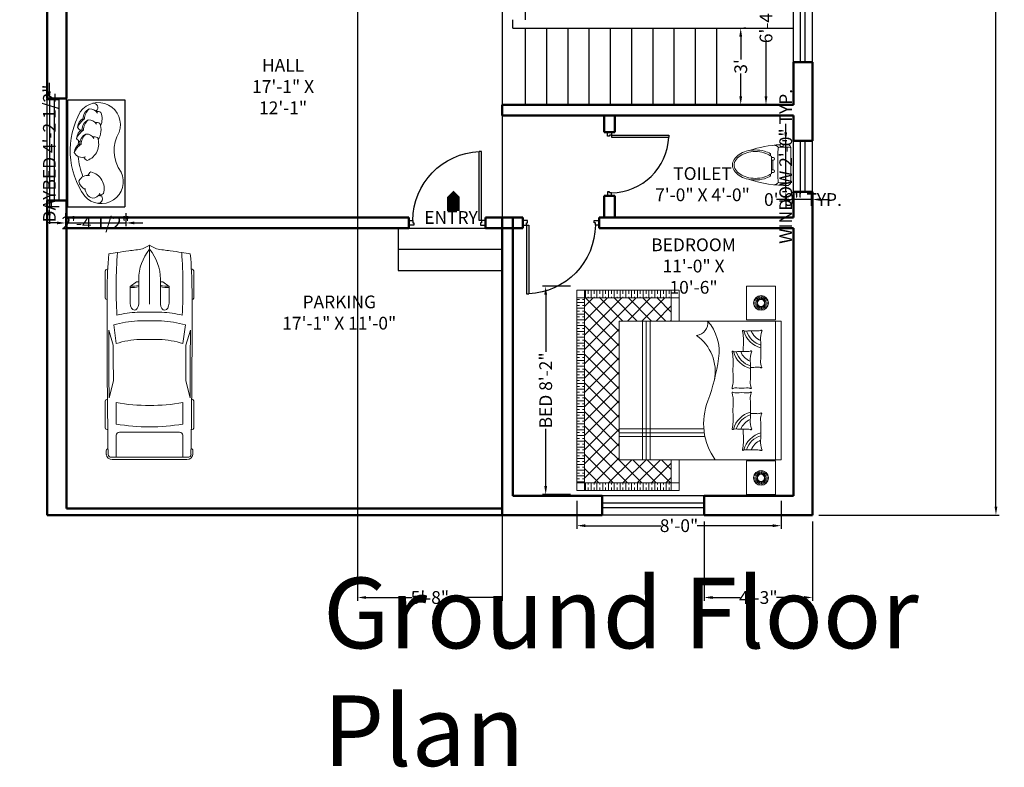
# Model space of a CAD drawing. Units: inches. Extents: x 234 to 707, y 260 to 1025.
# Tile 1 of 3: x 244 to 707, y 260 to 612. Entities that reach past the tile are written whole.
import ezdxf

# ---------------------------------------------------------------- set-up
doc = ezdxf.new("R2010")
doc.units = ezdxf.units.IN
doc.header["$MEASUREMENT"] = 0
for name, color, linetype, lineweight in [('A-ANNO-DIMS', 3, 'Continuous', 18), ('A-ANNO-SYMB', 3, 'Continuous', 18), ('A-ANNO-TEXT', 7, 'Continuous', 35), ('A-AREA-IDEN', 7, 'Continuous', 25), ('A-DOOR', 2, 'Continuous', 25), ('A-FLOR-FIXT', 9, 'Continuous', 18), ('A-FLOR-STRS', 4, 'Continuous', 25), ('A-FURN', 9, 'Continuous', 18), ('A-SITE-VEHI', 8, 'Continuous', 13), ('WALL', 7, 'Continuous', 50), ('WINDOW', 2, 'Continuous', 25)]:
    doc.layers.add(name, color=color, linetype=linetype, lineweight=lineweight)
doc.styles.get("Standard").update_dxf_attribs({"font": 'arial.ttf'})
doc.styles.add('YQ_DIM', font='SUPEROS.SHX', dxfattribs={"width": 0.8, "bigfont": 'HZDX.SHX'})
doc.dimstyles.new('yqi0', dxfattribs={"dimscale": 0, "dimtxt": 6, "dimasz": 4, "dimexe": 1.5, "dimexo": 3, "dimgap": 0.5, "dimtad": 0, "dimdec": 1, "dimdsep": 46, "dimlunit": 4, "dimtxsty": 'Standard', "dimcen": 0, "dimclrd": 256, "dimclre": 256, "dimclrt": 7, "dimadec": 1, "dimazin": 2, "dimtfac": 1, "dimtdec": 1, "dimtix": 1, "dimtmove": 2, "dimatfit": 2, "dimfxl": 1, "dimtolj": 1, "dimtzin": 0, "dimarcsym": 0})

# ---------------------------------------------------------------- blocks, each defined once
blk = doc.blocks.new('*D3')
at = {"layer": 'A-ANNO-DIMS', "color": 0, "lineweight": -2, "transparency": 16777216}
for p, q in [((620.21, 978.74), (705.01, 978.74)), ((703.51, 974.74), (703.51, 684.33)), ((703.51, 382.74), (703.51, 673.15)), ((620.21, 378.74), (705.01, 378.74))]:
    blk.add_line(p, q, dxfattribs=at)
at = {"layer": 'A-ANNO-DIMS', "color": 0, "transparency": 16777216}
for points in [[(702.84, 974.74), (704.17, 974.74), (703.51, 978.74)], [(702.84, 382.74), (704.17, 382.74), (703.51, 378.74)]]:
    blk.add_solid(points, dxfattribs=at)
at = {"layer": 'Defpoints', "color": 0, "transparency": 16777216}
for p in [(617.21, 978.74), (617.21, 378.74), (703.51, 378.74)]:
    blk.add_point(p, dxfattribs=at)
at = {"layer": 'A-ANNO-DIMS', "color": 0, "transparency": 16777216, "insert": (703.51, 678.74), "char_height": 6, "attachment_point": 5, "rotation": 90}
blk.add_mtext("\\A1;50'", dxfattribs=at)
blk = doc.blocks.new('DR_D01')
for p, q in [((-0.45, 0.93), (-0.42, 0.93)), ((-0.45, 0.03), (-0.45, 0.93)), ((-0.42, 0.03), (-0.42, 0.93)), ((-0.5, 0.03), (-0.42, 0.03)), ((-0.5, 0.03), (-0.5, -0.03)), ((-0.45, 0.03), (-0.45, 0)), ((-0.45, 0), (-0.435, 0)), ((-0.435, 0), (-0.435, -0.03)), ((0.435, 0), (0.435, -0.03)), ((0.45, 0), (0.435, 0)), ((0.45, 0.03), (0.45, 0)), ((0.5, 0.03), (0.45, 0.03)), ((0.5, -0.03), (0.5, 0.03)), ((-0.435, -0.03), (-0.5, -0.03)), ((0.435, -0.03), (0.5, -0.03))]:
    blk.add_line(p, q)
blk.add_arc((-0.46, 0.021), 0.91, 0.5915, 87.4664)
blk = doc.blocks.new('WD_WIN4')
for p, q in [((-0.5, 0.5), (0.5, 0.5)), ((-0.5, 0.12), (0.5, 0.12)), ((-0.5, -0.12), (0.5, -0.12)), ((-0.5, -0.5), (0.5, -0.5))]:
    blk.add_line(p, q)
blk = doc.blocks.new('yq_matong_01')
for p, q in [((0, 201), (0, -201)), ((20, 221), (139, 221)), ((252, 138), (252, 114)), ((216, 91), (238, 91)), ((216, 61), (238, 61)), ((223, 61), (223, -61)), ((238, 104), (238, -104)), ((216, -61), (238, -61)), ((216, -91), (238, -91)), ((252, -114), (252, -138)), ((20, -221), (139, -221)), ((97, -221), (97, -226)), ((97, -226), (132, -226)), ((132, -221), (132, -226))]:
    blk.add_line(p, q)
for centre, radius, start, end in [((55, 202), 54.8, 117.322, 181.8992), ((64, -1165), 1417, 71.4068, 91.3856), ((217, 161), 83.2, 95.4963, 139.9324), ((20, 201), 20, 90, 180), ((139, 201), 20, 2.3063, 90), ((-4840, 0), 5003, 357.6937, 2.3063), ((407, -123), 283, 105.2088, 123.2779), ((407, -123), 303, 105.2088, 120.5699), ((439, -242), 427, 74.7912, 105.2088), ((439, -242), 407, 74.7912, 105.2088), ((471, -123), 283, 56.7221, 74.7912), ((471, -123), 303, 56.7221, 74.7912), ((521, -47), 213, 32.2565, 56.7221), ((216, 76), 15, 90, 270), ((357, -47), 193, 123.2779, 128.1384), ((521, -47), 193, 32.2565, 56.7221), ((596, 0), 104, 360, 32.2565), ((596, 0), 124, 360, 32.2565), ((216, -76), 15, 90, 270), ((357, 47), 193, 231.8616, 236.7221), ((407, 123), 283, 236.7221, 254.7912), ((471, 123), 283, 285.2088, 303.2779), ((521, 47), 193, 303.2779, 327.7435), ((521, 47), 213, 303.2779, 327.7435), ((596, 0), 104, 327.7435, 360), ((596, 0), 124, 327.7435, 360), ((51, -204), 51.4, 175.687, 245.0918), ((20, -201), 20, 180, 270), ((157, -247), 63.1, 159.6834, 188.4939), ((72, -247), 63.1, 352.0944, 20.3166), ((64, 1165), 1417, 272.8967, 288.5932), ((139, -201), 20, 270, 357.6937), ((217, -161), 83.2, 220.0676, 264.5037), ((407, 123), 303, 239.4301, 254.7912), ((439, 242), 427, 254.7912, 285.2088), ((439, 242), 407, 254.7912, 285.2088), ((471, 123), 303, 285.2088, 303.2779), ((64, 1165), 1417, 268.6144, 271.2036), ((114, -226), 37, 237.5287, 304.2772)]:
    blk.add_arc(centre, radius, start, end)
blk = doc.blocks.new('20230926_Unit Plans$0$day bed')
blk.add_lwpolyline([(573.063, -307.537, -0.288423), (571.446, -307.621, -0.865931), (571.834, -306.876, 0.308297), (572.6, -306.836, -0.865931)], format="xyb", close=True)
for points in [[(571.715, -307.232, 0.201081), (571.457, -307.227, 0.121523), (571.44, -307.319, -7.115464)], [(571.979, -307.28, 0.24852), (571.668, -307.247, 0.121523), (571.651, -307.338, -7.115464)], [(572.665, -307.475, -0.165541), (572.598, -307.419, -0.425989), (573.013, -307.176, -0.121523), (573.04, -307.265, 7.115464)], [(571.587, -307.568, -0.306663), (571.391, -307.449, -0.30633), (571.474, -307.294, 0.872847)], [(571.798, -307.587, -0.306663), (571.602, -307.468, -0.30633), (571.685, -307.313, 0.872847)], [(572.071, -307.633, -0.306663), (571.875, -307.514, -0.30633), (571.958, -307.359, 0.872847)], [(572.317, -307.553, 0.165541), (572.379, -307.491, 0.425989), (571.941, -307.292, 0.121523), (571.924, -307.384, -7.115464)], [(572.919, -307.529, 0.306663), (573.101, -307.39, 0.30633), (573.003, -307.245, -0.872847)], [(571.743, -307.672, -0.14773), (571.586, -307.542, -0.213343), (571.391, -307.449, -0.178662)], [(571.804, -307.616, -0.116002), (571.743, -307.672, -0.249542), (571.573, -307.568, 9.61688)], [(571.955, -307.691, -0.14773), (571.798, -307.561, -0.213343), (571.602, -307.468, -0.178662)], [(572.019, -307.629, -0.125567), (571.955, -307.691, -0.249542), (571.784, -307.587, 9.61688)], [(572.227, -307.737, -0.14773), (572.07, -307.607, -0.213343), (571.875, -307.514, -0.178662)], [(572.31, -307.523, -0.356772), (572.227, -307.737, -0.249542), (572.057, -307.633, 9.61688)], [(572.669, -307.444, 0.356772), (572.774, -307.648, 0.249542), (572.933, -307.527, -9.61688)]]:
    blk.add_lwpolyline(points, format="xyb")
for centre, radius, start, end in [((573.116, -307.279), 0.084, 357.0539, 145.314), ((572.781, -307.22), 0.275, 348.5451, 359.7611), ((571.366, -307.37), 0.084, 40.6567, 188.9168), ((571.694, -307.277), 0.275, 186.2096, 192.1968), ((572.187, -306.294), 1.371, 274.7225, 291.4116), ((572.187, -306.294), 1.371, 262.2344, 265.3334)]:
    blk.add_arc(centre, radius, start, end)
at = {"layer": 'Defpoints', "ltscale": 0.1, "transparency": 33554687}
for p, q in [((571.219, -306.765), (573.269, -306.765)), ((571.219, -307.865), (571.219, -306.765)), ((573.269, -307.865), (573.269, -306.765)), ((571.219, -307.865), (573.269, -307.865))]:
    blk.add_line(p, q, dxfattribs=at)
blk = doc.blocks.new('*D15')
at = {"layer": 'A-ANNO-DIMS', "color": 0, "lineweight": -2, "transparency": 16777216}
for p, q in [((585.78, 607.74), (584.94, 607.74)), ((583.44, 603.74), (583.44, 593)), ((583.44, 575.74), (583.44, 586.48)), ((585.78, 571.74), (584.94, 571.74))]:
    blk.add_line(p, q, dxfattribs=at)
at = {"layer": 'A-ANNO-DIMS', "color": 0, "transparency": 16777216}
for points in [[(582.77, 603.74), (584.1, 603.74), (583.44, 607.74)], [(582.77, 575.74), (584.1, 575.74), (583.44, 571.74)]]:
    blk.add_solid(points, dxfattribs=at)
at = {"layer": 'Defpoints', "color": 0, "transparency": 16777216}
for p in [(582.78, 607.74), (583.44, 607.74), (582.78, 571.74)]:
    blk.add_point(p, dxfattribs=at)
at = {"layer": 'A-ANNO-DIMS', "color": 0, "transparency": 16777216, "insert": (583.44, 589.74), "char_height": 6, "attachment_point": 5, "rotation": 90}
blk.add_mtext("\\A1;3'", dxfattribs=at)
blk = doc.blocks.new('*D16')
at = {"layer": 'A-ANNO-DIMS', "color": 0, "lineweight": -2, "transparency": 16777216}
for p, q in [((598, 647.74), (596.84, 647.74)), ((595.34, 643.74), (595.34, 618.23)), ((595.34, 575.74), (595.34, 601.25)), ((598, 571.74), (596.84, 571.74))]:
    blk.add_line(p, q, dxfattribs=at)
at = {"layer": 'A-ANNO-DIMS', "color": 0, "transparency": 16777216}
for points in [[(594.67, 643.74), (596, 643.74), (595.34, 647.74)], [(594.67, 575.74), (596, 575.74), (595.34, 571.74)]]:
    blk.add_solid(points, dxfattribs=at)
at = {"layer": 'Defpoints', "color": 0, "transparency": 16777216}
for p in [(595, 647.74), (595.34, 647.74), (595, 571.74)]:
    blk.add_point(p, dxfattribs=at)
at = {"layer": 'A-ANNO-DIMS', "color": 0, "transparency": 16777216, "insert": (595.34, 609.74), "char_height": 6, "attachment_point": 5, "rotation": 90}
blk.add_mtext('\\A1;6\'-4"', dxfattribs=at)
blk = doc.blocks.new('*U19')
for p, q in [((536, 950), (536, 936)), ((1182, 988), (568, 988)), ((1214, 950), (1214, 950)), ((2235, 810), (1899, 912)), ((3412, 904), (3030, 807)), ((3440, 942), (3440, 950)), ((3472, 988), (4087, 988)), ((4119, 950), (4119, 934)), ((1779, 801), (2195, 746)), ((3516, 746), (3994, 746)), ((4179, 670), (4179, -670)), ((4736, 746), (4242, 746)), ((4736, -851), (4736, 851)), ((4785, -832), (4785, 832)), ((756, 241), (1313, 241)), ((816, 241), (816, 283)), ((820, 295), (918, 436)), ((918, 436), (1294, 436)), ((1496, -274), (1496, 274)), ((1690, -267), (1690, 267)), ((4736, -267), (4736, 267)), ((83, 156), (3, 10)), ((2102, 216), (2102, -216)), ((0, 0), (1313, 0)), ((3, -10), (83, -156)), ((756, -241), (1313, -241)), ((816, -241), (816, -283)), ((820, -295), (918, -436)), ((918, -436), (1294, -436)), ((2195, -746), (1779, -801)), ((2235, -810), (1899, -912)), ((3412, -904), (3030, -807)), ((3994, -746), (3516, -746)), ((4242, -746), (4736, -746)), ((536, -950), (536, -936)), ((1182, -988), (568, -988)), ((1214, -950), (1214, -950)), ((3440, -942), (3440, -950)), ((3472, -988), (4087, -988)), ((4119, -950), (4119, -934))]:
    blk.add_line(p, q)
for centre, major_axis, ratio, start_param, end_param in [((6757, -699), (0, 7958), 0.842304, 1.367076, 1.39176), ((1046, -12468), (0, 13417), 0.842304, 0.00281, 0.075598), ((568, 950), (0, -37.6), 0.842304, 3.141593, 4.712389), ((1638, -268113), (0, 269063), 0.842304, -0.013397, 0.002797), ((1182, 950), (0, 37.6), 0.842304, -1.570796, 0), ((1638, -268113), (0, -269025), 0.842304, 3.133765, 3.140441), ((3472, 950), (0, -37.6), 0.842304, 3.141593, 4.712389), ((4087, 950), (0, 37.6), 0.842304, -1.570796, 0), ((4588, 910), (0, 56.4), 0.842304, -0.013017, 1.249894), ((1638, -268131), (0, 269121), 0.842304, -0.013397, -0.013017), ((4673, 851), (0, -75.2), 0.842304, 1.570796, 3.128196), ((4673, 832), (0, -133), 0.842304, 1.570796, 3.128196), ((6583, -699), (0, -7755), 0.842304, 4.528606, 4.561838), ((952, -15087), (0, -15833), 0.842304, 3.096046, 3.200911), ((3414, 137), (0, -2280), 0.842304, 4.449482, 4.652344), ((3436, 137), (0, 2077), 0.842304, 1.245306, 1.50788), ((3800, 71), (0, -2021), 0.842304, 4.372215, 4.640744), ((2433, -93125), (0, -93935), 0.842304, 3.134049, 3.144098), ((434, 0), (0, 3734), 0.842304, 4.511394, 4.913384), ((912, 0), (0, 3734), 0.842304, 4.511394, 4.913384), ((4242, 670), (0, 75.2), 0.842304, 0, 1.570796), ((-5194, 1331), (0, -6374), 0.842304, 1.385369, 1.434372), ((756, -1185), (0, 1427), 0.842304, 0, 0.590319), ((832, 283), (0, 18.8), 0.842304, 0.879714, 1.570796), ((331, 432), (0, 696), 0.842304, 4.435146, 4.718221), ((361, 432), (0, 696), 0.842304, 4.435146, 4.718221), ((1290, 339), (161, -9), 0.603834, -1.395552, 1.581315), ((16, 0), (0, -18.8), 0.842304, 4.131459, 5.293319), ((-5194, -1331), (0, 6374), 0.842304, -1.434372, -1.385369), ((756, 1185), (0, 1427), 0.842304, 2.551274, 3.141593), ((3800, -71), (0, -2021), 0.842304, -1.499151, -1.230623), ((832, -283), (0, -18.8), 0.842304, 4.712389, 5.403472), ((331, -432), (0, -696), 0.842304, 1.564964, 1.848039), ((361, -432), (0, -696), 0.842304, 1.564964, 1.848039), ((3414, -137), (0, -2280), 0.842304, -1.510751, -1.307889), ((3436, -137), (0, -2077), 0.842304, -1.50788, -1.245306), ((6583, 699), (0, 7755), 0.842304, 1.721348, 1.754579), ((6757, 699), (0, 7958), 0.842304, 1.749832, 1.774517), ((952, 15087), (0, -15833), 0.842304, -0.059319, 0.045547), ((2433, 93125), (0, -93935), 0.842304, -0.002505, 0.007544), ((4242, -670), (0, -75.2), 0.842304, 4.712389, 6.283185), ((4673, -851), (0, 75.2), 0.842304, 3.15499, 4.712389), ((4673, -832), (0, -133), 0.842304, 0.013397, 1.570796), ((1046, 12468), (0, -13417), 0.842304, -0.075598, -0.00281), ((568, -950), (0, 37.6), 0.842304, 1.570796, 3.141593), ((1638, 268113), (0, 269063), 0.842304, 3.138796, 3.15499), ((1182, -950), (0, -37.6), 0.842304, 0, 1.570796), ((1638, 268113), (0, -269025), 0.842304, 0.001152, 0.007828), ((3472, -950), (0, -37.6), 0.842304, -1.570796, 0), ((4087, -950), (0, 37.6), 0.842304, 3.141593, 4.712389), ((4588, -910), (0, -56.4), 0.842304, -1.249894, 0.013017), ((1638, 268131), (0, 269121), 0.842304, 3.15461, 3.15499)]:
    blk.add_ellipse(centre, major_axis=major_axis, ratio=ratio, start_param=start_param, end_param=end_param)
at = {"extrusion": (0, 0, -1)}
blk.add_ellipse((1290, -339), major_axis=(161, 9), ratio=0.603834, start_param=-1.395552, end_param=1.581315, dxfattribs=at)
blk = doc.blocks.new('BED')
h = blk.add_hatch()
h.set_pattern_fill('TRANS', color=256, scale=12, style=0)
h.set_pattern_definition([(360, (4433.967, -9715.0492), (1e-15, 3), []), (360, (4433.967, -9713.5492), (1e-15, 3), [1.5, -1.5])])
h.paths.add_polyline_path([(48, -103), (52, -103), (52, -58), (48, -58)])
h.paths.add_polyline_path([(-48, -58), (-52, -58), (-52, -103), (-48, -103)])
h = blk.add_hatch()
h.set_pattern_fill('ANSI37', color=256, scale=42, angle=-90, style=0)
h.set_pattern_definition([(315, (7787.1367, 4477.8466), (3.7123106, 3.7123106), []), (45, (7787.1367, 4477.8466), (-3.7123106, 3.7123106), [])])
h.paths.add_polyline_path([(-36, -85), (-36, -58), (-48, -58), (-48, -103), (48, -103), (48, -58), (36, -58), (36, -85)])
h = blk.add_hatch()
h.set_pattern_fill('TRANS', color=256, scale=12, angle=-90, style=0)
h.set_pattern_definition([(270, (4433.967, -9715.0492), (3, -1e-15), []), (270, (4435.467, -9715.0492), (3, -1e-15), [1.5, -1.5])])
h.paths.add_polyline_path([(48, -107), (48, -103), (-48, -103), (-48, -107)])
for p, q in [((-54, -4), (-54, -19)), ((-36.64, -4), (-54, -4)), ((-36.64, -4), (-36.64, -19)), ((-36, -1), (36, -1)), ((-36, -85), (-36, -1)), ((-36, -4), (36, -4)), ((36, -1), (36, -85)), ((36.64, -4), (36.64, -19)), ((36.64, -4), (54, -4)), ((54, -4), (54, -19)), ((-47.07, -10.7), (-48.9, -9.89)), ((-46.88, -10.37), (-48.5, -9.2)), ((-46.62, -10.08), (-47.96, -8.6)), ((-46.31, -9.86), (-47.31, -8.13)), ((-45.96, -9.7), (-46.58, -7.8)), ((-45.58, -9.62), (-45.8, -7.63)), ((-45.2, -9.62), (-45, -7.63)), ((-44.82, -9.7), (-44.21, -7.79)), ((-44.47, -9.85), (-43.48, -8.12)), ((-44.16, -10.08), (-42.83, -8.59)), ((-43.9, -10.36), (-42.29, -9.18)), ((-43.71, -10.7), (-41.89, -9.88)), ((43.71, -10.7), (41.89, -9.88)), ((43.9, -10.36), (42.29, -9.18)), ((44.16, -10.08), (42.83, -8.59)), ((44.47, -9.85), (43.48, -8.12)), ((44.82, -9.7), (44.21, -7.79)), ((45.2, -9.62), (45, -7.63)), ((45.58, -9.62), (45.8, -7.63)), ((45.96, -9.7), (46.58, -7.8)), ((46.31, -9.86), (47.31, -8.13)), ((46.62, -10.08), (47.96, -8.6)), ((46.88, -10.37), (48.5, -9.2)), ((47.07, -10.7), (48.9, -9.89)), ((-47.23, -11.45), (-49.23, -11.45)), ((-47.19, -11.07), (-49.14, -10.66)), ((-47.19, -11.83), (-49.14, -12.25)), ((-47.07, -12.2), (-48.89, -13.01)), ((-46.87, -12.53), (-48.49, -13.71)), ((-46.62, -12.81), (-47.95, -14.3)), ((-46.3, -13.04), (-47.3, -14.77)), ((-45.95, -13.2), (-46.57, -15.1)), ((-45.58, -13.27), (-45.78, -15.26)), ((-45.19, -13.27), (-44.98, -15.26)), ((-44.82, -13.19), (-44.2, -15.09)), ((-44.47, -13.04), (-43.46, -14.77)), ((-44.16, -12.81), (-42.82, -14.29)), ((-43.9, -12.52), (-42.28, -13.7)), ((-43.71, -12.19), (-41.88, -13)), ((-43.59, -11.06), (-41.64, -10.64)), ((-43.59, -11.83), (-41.63, -12.24)), ((-43.55, -11.44), (-41.55, -11.44)), ((43.55, -11.44), (41.55, -11.44)), ((43.59, -11.83), (41.63, -12.24)), ((43.59, -11.06), (41.64, -10.64)), ((43.71, -12.19), (41.88, -13)), ((43.9, -12.52), (42.28, -13.7)), ((44.16, -12.81), (42.82, -14.29)), ((44.47, -13.04), (43.46, -14.77)), ((44.82, -13.19), (44.2, -15.09)), ((45.19, -13.27), (44.98, -15.26)), ((45.58, -13.27), (45.78, -15.26)), ((45.95, -13.2), (46.57, -15.1)), ((46.3, -13.04), (47.3, -14.77)), ((46.62, -12.81), (47.95, -14.3)), ((46.87, -12.53), (48.49, -13.71)), ((47.07, -12.2), (48.89, -13.01)), ((47.19, -11.07), (49.14, -10.66)), ((47.19, -11.83), (49.14, -12.25)), ((47.23, -11.45), (49.23, -11.45)), ((-36.64, -19), (-54, -19)), ((36.64, -19), (54, -19)), ((24, -85), (24, -40.55)), ((20, -85), (20, -41.14)), ((22, -85), (22, -40.91)), ((-52, -54), (-52, -107)), ((-52, -54), (-36, -54)), ((-48, -54), (-48, -107)), ((36, -54), (52, -54)), ((48, -54), (48, -107)), ((52, -54), (52, -107)), ((-52, -58), (-36, -58)), ((36, -58), (52, -58)), ((36, -69), (-36, -69)), ((36, -71), (-36, -71)), ((36, -73), (-36, -73)), ((36, -85), (-36, -85)), ((-52, -103), (52, -103)), ((-52, -107), (52, -107))]:
    blk.add_line(p, q)
for centre, radius in [((-45.39, -11.45), 3.84), ((-45.39, -11.45), 1.84), ((45.39, -11.45), 3.84), ((45.39, -11.45), 1.84)]:
    blk.add_circle(centre, radius)
for centre, radius, start, end in [((-30.92, -11.24), 0.328, 35.8976, 208.6272), ((-42.38, -17.5), 12.73, 27.1629, 28.6272), ((-44.37, -13.89), 13.5, 357.4804, 9.3956), ((10.15, -16.29), 41.07, 177.4804, 184.5075), ((-33.8, -8.61), 8.46, 289.8695, 338.9843), ((-33.8, -8.61), 12.06, 283.8498, 346.0842), ((-33.8, -8.61), 10.71, 286.0319, 344.1205), ((-26.84, 0.13), 11.82, 251.1782, 273.3982), ((-20.92, -99.64), 88.13, 86.2964, 93.3982), ((-14.79, -4.98), 6.73, 266.2964, 294.303), ((-8.24, -13.16), 3.86, 159.0146, 186.273), ((-36.64, -16.28), 24.71, 358.5721, 6.273), ((-11.92, -11.33), 0.242, 335.7259, 114.303), ((-5.69, -14.14), 6.59, 155.7259, 159.0146), ((11.92, -11.33), 0.242, 65.697, 204.2741), ((5.69, -14.14), 6.59, 20.9854, 24.2741), ((8.24, -13.16), 3.86, 353.727, 20.9854), ((36.64, -16.28), 24.71, 173.727, 181.4279), ((14.79, -4.98), 6.73, 245.697, 273.7036), ((20.92, -99.64), 88.13, 86.6018, 93.7036), ((33.8, -8.61), 12.06, 193.9158, 256.1502), ((33.8, -8.61), 10.71, 195.8795, 253.9681), ((33.8, -8.61), 8.46, 201.0157, 250.1305), ((26.84, 0.13), 11.82, 266.6018, 288.8218), ((30.92, -11.24), 0.328, 331.3728, 144.1024), ((-10.15, -16.29), 41.07, 355.4925, 2.5196), ((44.37, -13.89), 13.5, 170.6044, 182.5196), ((42.38, -17.5), 12.73, 151.3728, 152.8371), ((-32.72, -19.65), 1.93, 327.6219, 339.2246), ((-32.67, -19.67), 1.88, 339.2246, 4.5075), ((-20.16, -16.62), 0.328, 35.8976, 208.6272), ((-31.62, -22.87), 12.73, 27.1629, 28.6272), ((-33.61, -19.26), 13.5, 357.4804, 9.3956), ((-23.04, -13.99), 8.46, 289.8695, 338.9843), ((20.91, -21.66), 41.07, 177.4804, 184.5075), ((-23.04, -13.99), 12.06, 283.8498, 346.0842), ((-23.04, -13.99), 10.71, 286.0319, 344.1205), ((-16.08, -5.24), 11.82, 251.1782, 273.3982), ((-10.15, -105.01), 88.13, 86.2964, 93.3982), ((-4.03, -10.35), 6.73, 266.2964, 294.303), ((2.52, -18.53), 3.86, 159.0146, 186.273), ((-25.88, -21.66), 24.71, 354.3784, 6.273), ((-1.16, -16.7), 0.242, 335.7259, 114.303), ((5.07, -19.51), 6.59, 155.7259, 159.0146), ((1.16, -16.7), 0.242, 65.697, 204.2741), ((-5.07, -19.51), 6.59, 20.9854, 24.2741), ((-2.52, -18.53), 3.86, 353.727, 20.9854), ((25.88, -21.66), 24.71, 173.727, 185.6216), ((4.03, -10.35), 6.73, 245.697, 273.7036), ((10.15, -105.01), 88.13, 86.6018, 93.7036), ((23.04, -13.99), 12.06, 193.9158, 256.1502), ((23.04, -13.99), 10.71, 195.8795, 253.9681), ((23.04, -13.99), 8.46, 201.0157, 250.1305), ((16.08, -5.24), 11.82, 266.6018, 288.8218), ((20.16, -16.62), 0.328, 331.3728, 144.1024), ((-20.91, -21.66), 41.07, 355.4925, 2.5196), ((33.61, -19.26), 13.5, 170.6044, 182.5196), ((31.62, -22.87), 12.73, 151.3728, 152.8371), ((32.67, -19.67), 1.88, 175.4925, 200.7754), ((32.72, -19.65), 1.93, 200.7754, 212.3781), ((-30.88, -20.82), 0.25, 147.6219, 311.9343), ((-25.16, -53.53), 33, 93.5164, 99.6766), ((-25.27, -51.86), 31.33, 86.4836, 93.5164), ((-21.12, 15.68), 36.34, 266.4836, 271.5234), ((-21.91, -25.04), 1.88, 339.2246, 4.5075), ((2.55, -24.46), 3.86, 174.3784, 204.7617), ((-2.55, -24.46), 3.86, 335.2383, 5.6216), ((21.91, -25.04), 1.88, 175.4925, 200.7754), ((21.12, 15.68), 36.34, 268.4766, 273.5164), ((25.27, -51.86), 31.33, 86.4836, 93.5164), ((25.16, -53.53), 33, 80.3234, 86.4836), ((30.88, -20.82), 0.25, 228.0657, 32.3781), ((-20.12, -26.19), 0.25, 147.6219, 311.9343), ((-21.96, -25.02), 1.93, 327.6219, 339.2246), ((-14.4, -58.9), 33, 93.5164, 99.6766), ((-14.51, -57.23), 31.33, 86.4836, 93.5164), ((-10.35, 10.3), 36.34, 266.4836, 275.306), ((-5.78, -38.98), 13.15, 77.9645, 95.306), ((2.5, -0.17), 26.53, 257.9645, 261.9243), ((-1.09, -26.25), 0.228, 231.9005, 52.8902), ((1.09, -26.25), 0.228, 127.1098, 308.0995), ((-2.5, -0.17), 26.53, 278.0757, 282.0355), ((5.78, -38.98), 13.15, 84.694, 102.0355), ((10.35, 10.3), 36.34, 264.694, 273.5164), ((14.51, -57.23), 31.33, 86.4836, 93.5164), ((14.4, -58.9), 33, 80.3234, 86.4836), ((20.12, -26.19), 0.25, 228.0657, 32.3781), ((21.96, -25.02), 1.93, 200.7754, 212.3781), ((-20.27, -56.85), 23.66, 81.0857, 131.6581), ((-9.91, -57.83), 22.61, 78.6456, 145.1521), ((-32.56, -143.87), 111.55, 70.0977, 81.7735), ((17.27, -9.21), 32.05, 248.2778, 305.7663), ((-34.97, -45.63), 6.55, 6.3172, 99.0807)]:
    blk.add_arc(centre, radius, start, end)
blk = doc.blocks.new('*D25')
at = {"layer": 'A-ANNO-DIMS', "lineweight": -2, "transparency": 16777216}
for p, q in [((604.61, 558.74), (604.61, 562.74)), ((605.21, 554.74), (603.11, 554.74)), ((604.61, 530.74), (604.61, 554.74)), ((605.21, 530.74), (603.11, 530.74)), ((604.61, 526.74), (604.61, 522.74))]:
    blk.add_line(p, q, dxfattribs=at)
at = {"layer": 'A-ANNO-DIMS', "transparency": 16777216}
for points in [[(603.95, 558.74), (605.28, 558.74), (604.61, 554.74)], [(603.95, 526.74), (605.28, 526.74), (604.61, 530.74)]]:
    blk.add_solid(points, dxfattribs=at)
at = {"layer": 'Defpoints', "color": 0, "transparency": 16777216}
for p in [(604.61, 554.74), (608.21, 554.74), (608.21, 530.74)]:
    blk.add_point(p, dxfattribs=at)
at = {"layer": 'A-ANNO-DIMS', "color": 7, "transparency": 16777216, "insert": (604.61, 542.74), "char_height": 6, "attachment_point": 5, "rotation": 90}
blk.add_mtext('\\A1;WINDOW 2\'-0" TYP.', dxfattribs=at)
blk = doc.blocks.new('*D26')
at = {"layer": 'A-ANNO-DIMS', "lineweight": -2, "transparency": 16777216}
for p, q in [((604.21, 527.14), (600.21, 527.14)), ((608.21, 527.74), (608.21, 525.64)), ((617.21, 527.14), (608.21, 527.14)), ((617.21, 527.74), (617.21, 525.64)), ((621.21, 527.14), (625.21, 527.14))]:
    blk.add_line(p, q, dxfattribs=at)
at = {"layer": 'A-ANNO-DIMS', "transparency": 16777216}
for points in [[(604.21, 527.81), (604.21, 526.47), (608.21, 527.14)], [(621.21, 527.81), (621.21, 526.47), (617.21, 527.14)]]:
    blk.add_solid(points, dxfattribs=at)
at = {"layer": 'Defpoints', "color": 0, "transparency": 16777216}
for p in [(608.21, 530.74), (617.21, 530.74), (608.21, 527.14)]:
    blk.add_point(p, dxfattribs=at)
at = {"layer": 'A-ANNO-DIMS', "color": 7, "transparency": 16777216, "insert": (612.71, 527.14), "char_height": 6, "attachment_point": 5}
blk.add_mtext('\\A1;0\'-9" TYP.', dxfattribs=at)
blk = doc.blocks.new('*D35')
at = {"layer": 'A-ANNO-DIMS', "lineweight": -2, "transparency": 16777216}
for p, q in [((503.37, 486.32), (490.19, 486.32)), ((491.69, 482.32), (491.69, 455.49)), ((491.69, 392.41), (491.69, 419.24)), ((503.37, 388.41), (490.19, 388.41))]:
    blk.add_line(p, q, dxfattribs=at)
at = {"layer": 'A-ANNO-DIMS', "transparency": 16777216}
for points in [[(491.02, 482.32), (492.35, 482.32), (491.69, 486.32)], [(491.02, 392.41), (492.35, 392.41), (491.69, 388.41)]]:
    blk.add_solid(points, dxfattribs=at)
at = {"layer": 'Defpoints', "color": 0, "transparency": 16777216}
for p in [(506.37, 486.32), (491.69, 388.41), (506.37, 388.41)]:
    blk.add_point(p, dxfattribs=at)
at = {"layer": 'A-ANNO-DIMS', "color": 7, "transparency": 16777216, "insert": (491.69, 437.37), "char_height": 6, "attachment_point": 5, "rotation": 90}
blk.add_mtext('\\A1;BED 8\'-2"', dxfattribs=at)
blk = doc.blocks.new('*D36')
at = {"layer": 'A-ANNO-DIMS', "lineweight": -2, "transparency": 16777216}
for p, q in [((506.37, 385.41), (506.37, 372.23)), ((602.47, 385.41), (602.47, 372.23)), ((510.37, 373.73), (545.94, 373.73)), ((598.47, 373.73), (562.9, 373.73))]:
    blk.add_line(p, q, dxfattribs=at)
at = {"layer": 'A-ANNO-DIMS', "transparency": 16777216}
for points in [[(510.37, 374.39), (510.37, 373.06), (506.37, 373.73)], [(598.47, 374.39), (598.47, 373.06), (602.47, 373.73)]]:
    blk.add_solid(points, dxfattribs=at)
at = {"layer": 'Defpoints', "color": 0, "transparency": 16777216}
for p in [(506.37, 388.41), (602.47, 388.41), (602.47, 373.73)]:
    blk.add_point(p, dxfattribs=at)
at = {"layer": 'A-ANNO-DIMS', "color": 7, "transparency": 16777216, "insert": (554.42, 373.73), "char_height": 6, "attachment_point": 5}
blk.add_mtext('\\A1;8\'-0"', dxfattribs=at)
blk = doc.blocks.new('*D43')
at = {"layer": 'A-ANNO-DIMS', "lineweight": -2, "transparency": 16777216}
for p, q in [((258.2, 577.98), (258.2, 581.98)), ((262.75, 573.98), (256.7, 573.98)), ((258.2, 573.98), (258.2, 523.67)), ((262.75, 523.67), (256.7, 523.67)), ((258.2, 519.67), (258.2, 515.67))]:
    blk.add_line(p, q, dxfattribs=at)
at = {"layer": 'A-ANNO-DIMS', "transparency": 16777216}
for points in [[(257.53, 577.98), (258.86, 577.98), (258.2, 573.98)], [(257.53, 519.67), (258.86, 519.67), (258.2, 523.67)]]:
    blk.add_solid(points, dxfattribs=at)
at = {"layer": 'Defpoints', "color": 0, "transparency": 16777216}
for p in [(265.75, 573.98), (258.2, 523.67), (265.75, 523.67)]:
    blk.add_point(p, dxfattribs=at)
at = {"layer": 'A-ANNO-DIMS', "color": 7, "transparency": 16777216, "insert": (258.2, 548.83), "char_height": 6, "attachment_point": 5, "rotation": 90}
blk.add_mtext('\\A1;DAYBED 4\'-2 1/2"', dxfattribs=at)
blk = doc.blocks.new('*D44')
at = {"layer": 'A-ANNO-DIMS', "lineweight": -2, "transparency": 16777216}
for p, q in [((265.75, 520.67), (265.75, 514.62)), ((294.24, 520.67), (294.24, 514.62)), ((261.75, 516.12), (257.75, 516.12)), ((265.75, 516.12), (294.24, 516.12)), ((298.24, 516.12), (302.24, 516.12))]:
    blk.add_line(p, q, dxfattribs=at)
at = {"layer": 'A-ANNO-DIMS', "transparency": 16777216}
for points in [[(261.75, 516.79), (261.75, 515.46), (265.75, 516.12)], [(298.24, 516.79), (298.24, 515.46), (294.24, 516.12)]]:
    blk.add_solid(points, dxfattribs=at)
at = {"layer": 'Defpoints', "color": 0, "transparency": 16777216}
for p in [(265.75, 523.67), (294.24, 523.67), (294.24, 516.12)]:
    blk.add_point(p, dxfattribs=at)
at = {"layer": 'A-ANNO-DIMS', "color": 7, "transparency": 16777216, "insert": (279.99, 516.12), "char_height": 6, "attachment_point": 5}
blk.add_mtext('\\A1;2\'-4 1/2"', dxfattribs=at)
blk = doc.blocks.new('*D53')
at = {"layer": 'A-ANNO-DIMS', "lineweight": -2, "transparency": 16777216}
for p, q in [((566.21, 375.74), (566.21, 338.44)), ((617.21, 375.74), (617.21, 338.44)), ((570.21, 339.94), (583.12, 339.94)), ((613.21, 339.94), (600.31, 339.94))]:
    blk.add_line(p, q, dxfattribs=at)
at = {"layer": 'A-ANNO-DIMS', "transparency": 16777216}
for points in [[(570.21, 340.61), (570.21, 339.27), (566.21, 339.94)], [(613.21, 340.61), (613.21, 339.27), (617.21, 339.94)]]:
    blk.add_solid(points, dxfattribs=at)
at = {"layer": 'Defpoints', "color": 0, "transparency": 16777216}
for p in [(566.21, 378.74), (617.21, 378.74), (617.21, 339.94)]:
    blk.add_point(p, dxfattribs=at)
at = {"layer": 'A-ANNO-DIMS', "color": 7, "transparency": 16777216, "insert": (591.71, 339.94), "char_height": 6, "attachment_point": 5}
blk.add_mtext('\\A1;4\'-3"', dxfattribs=at)
blk = doc.blocks.new('*D54')
at = {"layer": 'A-ANNO-DIMS', "lineweight": -2, "transparency": 16777216}
for p, q in [((403.21, 899.74), (403.21, 338.44)), ((471.21, 899.74), (471.21, 338.44)), ((407.21, 339.94), (428.74, 339.94)), ((467.21, 339.94), (445.69, 339.94))]:
    blk.add_line(p, q, dxfattribs=at)
at = {"layer": 'A-ANNO-DIMS', "transparency": 16777216}
for points in [[(407.21, 340.61), (407.21, 339.27), (403.21, 339.94)], [(467.21, 340.61), (467.21, 339.27), (471.21, 339.94)]]:
    blk.add_solid(points, dxfattribs=at)
at = {"layer": 'Defpoints', "color": 0, "transparency": 16777216}
for p in [(403.21, 902.74), (471.21, 902.74), (471.21, 339.94)]:
    blk.add_point(p, dxfattribs=at)
at = {"layer": 'A-ANNO-DIMS', "color": 7, "transparency": 16777216, "insert": (437.21, 339.94), "char_height": 6, "attachment_point": 5}
blk.add_mtext('\\A1;5\'-8"', dxfattribs=at)

msp = doc.modelspace()

# ---------------------------------------------------------------- linework, layer by layer
at = {"layer": 'A-ANNO-SYMB'}
msp.add_lwpolyline([(448.28, 531.35, 0, 12, 0), (448.28, 525.35, 6, 6, 0), (448.28, 521.75, 6, 6, 0)], format="xyseb", dxfattribs=at)
at = {"layer": 'A-FLOR-STRS'}
for p, q in [((482.21, 611.74), (482.21, 647.74)), ((476.21, 607.74), (476.21, 611.74)), ((476.21, 607.74), (608.21, 607.74)), ((482.21, 571.74), (482.21, 607.74)), ((492.21, 571.74), (492.21, 607.74)), ((502.21, 571.74), (502.21, 607.74)), ((512.21, 571.74), (512.21, 607.74)), ((522.21, 571.74), (522.21, 607.74)), ((532.21, 571.74), (532.21, 607.74)), ((542.21, 571.74), (542.21, 607.74)), ((552.21, 571.74), (552.21, 607.74)), ((562.21, 571.74), (562.21, 607.74)), ((572.21, 571.74), (572.21, 607.74)), ((422.27, 513.74), (422.27, 493.74)), ((427.34, 513.74), (463.34, 513.74)), ((422.27, 503.74), (471.21, 503.74)), ((422.27, 493.74), (427.34, 493.74)), ((427.34, 493.74), (471.21, 493.74))]:
    msp.add_line(p, q, dxfattribs=at)
at = {"layer": 'WALL'}
for p, q in [((257.21, 574.62), (257.21, 716.87)), ((266.21, 574.62), (266.21, 716.87)), ((608.21, 571.74), (608.21, 591.74)), ((608.21, 591.74), (617.21, 591.74)), ((617.21, 554.74), (617.21, 591.74)), ((266.21, 574.62), (257.21, 574.62)), ((471.21, 571.74), (608.21, 571.74)), ((471.21, 566.74), (471.21, 571.74)), ((471.21, 566.74), (608.21, 566.74)), ((519.21, 558.87), (519.21, 566.74)), ((524.21, 558.87), (524.21, 566.74)), ((608.21, 554.74), (608.21, 566.74)), ((524.21, 558.87), (519.21, 558.87)), ((608.21, 554.74), (617.21, 554.74)), ((519.21, 518.74), (519.21, 528.87)), ((524.21, 528.87), (519.21, 528.87)), ((524.21, 518.74), (524.21, 528.87)), ((608.21, 518.74), (608.21, 530.74)), ((608.21, 530.74), (617.21, 530.74)), ((617.21, 378.74), (617.21, 530.74)), ((257.21, 378.74), (257.21, 526.62)), ((266.21, 526.62), (257.21, 526.62)), ((266.21, 381.74), (266.21, 526.62)), ((266.21, 518.74), (427.34, 518.74)), ((427.34, 518.74), (427.34, 513.74)), ((463.34, 518.74), (476.21, 518.74)), ((463.34, 518.74), (463.34, 513.74)), ((471.21, 378.74), (471.21, 518.74)), ((476.21, 387.74), (476.21, 518.74)), ((476.21, 518.74), (480.87, 518.74)), ((480.87, 513.74), (480.87, 518.74)), ((516.87, 518.74), (608.21, 518.74)), ((516.87, 513.74), (516.87, 518.74)), ((266.21, 513.74), (427.34, 513.74)), ((463.34, 513.74), (476.21, 513.74)), ((476.21, 513.74), (480.87, 513.74)), ((516.87, 513.74), (608.21, 513.74)), ((608.21, 387.74), (608.21, 513.74)), ((476.21, 387.74), (518.21, 387.74)), ((518.21, 387.74), (518.21, 378.74)), ((566.21, 387.74), (608.21, 387.74)), ((566.21, 387.74), (566.21, 378.74)), ((266.21, 381.74), (471.21, 381.74)), ((257.21, 378.74), (518.21, 378.74)), ((566.21, 378.74), (617.21, 378.74))]:
    msp.add_line(p, q, dxfattribs=at)

# ---------------------------------------------------------------- block references
at = {"layer": 'A-DOOR'}
for p, xscale, yscale, zscale, rotation in [((521.71, 543.87), 30, 30, 30, 270.0000000000002), ((445.34, 516.24), 36, -36, 36, 180.0000000000001)]:
    msp.add_blockref('DR_D01', p, dxfattribs=dict(at, xscale=xscale, yscale=yscale, zscale=zscale, rotation=rotation))
at = {"layer": 'A-DOOR', "xscale": 36, "yscale": -36, "zscale": 36}
msp.add_blockref('DR_D01', (498.87, 516.24), dxfattribs=at)
at = {"layer": 'A-FLOR-FIXT', "xscale": 0.0381663584185813, "yscale": 0.0381663584185813, "zscale": 0.0381663584185813, "rotation": 180}
msp.add_blockref('yq_matong_01', (607.08, 543.4), dxfattribs=at)
at = {"layer": 'A-FURN', "rotation": 270}
for name, p, xscale, yscale, zscale in [('20230926_Unit Plans$0$day bed', (7822.98, 14593.94), 24.54391766436544, 24.54391766436544, 24.54391766436544), ('BED', (603.37, 437.37), 0.9065569866853559, 0.9065569866853559, 0.9065569866853559)]:
    msp.add_blockref(name, p, dxfattribs=dict(at, xscale=xscale, yscale=yscale, zscale=zscale))
at = {"layer": 'A-SITE-VEHI', "xscale": 0.0210571382333109, "yscale": 0.0210571382333109, "zscale": 0.0210571382333109, "rotation": 270}
msp.add_blockref('*U19', (305.33, 505.64), dxfattribs=at)
at = {"layer": 'WINDOW'}
for p, xscale, yscale, zscale, rotation in [((612.71, 609.74), 36, 9.000000000001023, 36, 90), ((261.71, 550.62), 48, 9.000000000001535, 48, 89.99999999999973), ((612.71, 542.74), 24, 9.000000000000568, 24, 90), ((542.21, 383.24), 48, 9.000000000002387, 48, 179.9999999999997)]:
    msp.add_blockref('WD_WIN4', p, dxfattribs=dict(at, xscale=xscale, yscale=yscale, zscale=zscale, rotation=rotation))

# ---------------------------------------------------------------- texts
at = {"layer": 'A-ANNO-TEXT', "insert": (387.01, 349.27), "char_height": 33.2325, "width": 310.2889, "attachment_point": 1, "style": 'YQ_DIM'}
msp.add_mtext('Ground Floor Plan', dxfattribs=at)
at = {"layer": 'A-AREA-IDEN', "char_height": 13.7795, "attachment_point": 1, "style": 'YQ_DIM'}
for s, insert, width in [('\\pxqc;{\\H0.43543x;HALL\\P17\'-1" X 12\'-1"}', (343.01, 593.3), 50.2899), ('\\pxqc;{\\H0.43543x;TOILET\\P7\'-0" X 4\'-0"}', (540.32, 542.37), 50.2899), ('\\pxqc;{\\H0.43543x;ENTRY}', (435.48, 521.7), 23.3591), ('\\pxqc;{\\H0.43543x;BEDROOM\\P11\'-0" X 10\'-6"}', (536.11, 508.85), 50.2899), ('\\pxqc;{\\H0.43543x;PARKING\\P17\'-1" X 11\'-0"}', (364.54, 481.98), 60.0872)]:
    msp.add_mtext(s, dxfattribs=dict(at, insert=insert, width=width))

# ---------------------------------------------------------------- dimensions: what is measured, and where the dimension line sits
at = {"layer": 'A-ANNO-DIMS'}
for p1, p2, distance, picture, middle in [((617.21, 978.74), (617.21, 378.74), 86.29, '*D3', (703.51, 678.74)), ((595, 571.74), (595, 647.74), -0.33, '*D16', (595.34, 609.74)), ((582.78, 571.74), (582.78, 607.74), -0.66, '*D15', (583.44, 589.74))]:
    dim = msp.add_aligned_dim(p1=p1, p2=p2, distance=distance, dimstyle='yqi0', override={"dimscale": 1, "dimclrd": 0, "dimclre": 0, "dimclrt": 0}, dxfattribs=at)
    dim.commit()
    dim.dimension.update_dxf_attribs({"geometry": picture, "text_midpoint": middle})
for base, p1, p2, picture, middle in [((471.21, 339.94), (403.21, 902.74), (471.21, 902.74), '*D54', (437.21, 339.94)), ((294.24, 516.12), (265.75, 523.67), (294.24, 523.67), '*D44', (279.99, 516.12)), ((602.47, 373.73), (506.37, 388.41), (602.47, 388.41), '*D36', (554.42, 373.73)), ((617.21, 339.94), (566.21, 378.74), (617.21, 378.74), '*D53', (591.71, 339.94))]:
    dim = msp.add_linear_dim(base=base, p1=p1, p2=p2, dimstyle='yqi0', override={"dimscale": 1, "dimzin": 1, "dimfrac": 2}, dxfattribs=at)
    dim.commit()
    dim.dimension.update_dxf_attribs({"geometry": picture, "text_midpoint": middle})
for base, p1, p2, angle, text, picture, middle in [((258.2, 523.67), (265.75, 573.98), (265.75, 523.67), 270, 'DAYBED <>', '*D43', (258.2, 548.83)), ((604.61, 554.74), (608.21, 530.74), (608.21, 554.74), 90, 'WINDOW <> TYP.', '*D25', (604.61, 542.74)), ((608.21, 527.14), (617.21, 530.74), (608.21, 530.74), 180, '<> TYP.', '*D26', (612.71, 527.14)), ((491.69, 388.41), (506.37, 486.32), (506.37, 388.41), 270, 'BED <>', '*D35', (491.69, 437.37))]:
    dim = msp.add_linear_dim(base=base, p1=p1, p2=p2, angle=angle, text=text, dimstyle='yqi0', override={"dimscale": 1, "dimzin": 1, "dimfrac": 2}, dxfattribs=at)
    dim.commit()
    dim.dimension.update_dxf_attribs({"geometry": picture, "text_midpoint": middle})

doc.saveas('drawing.dxf')
